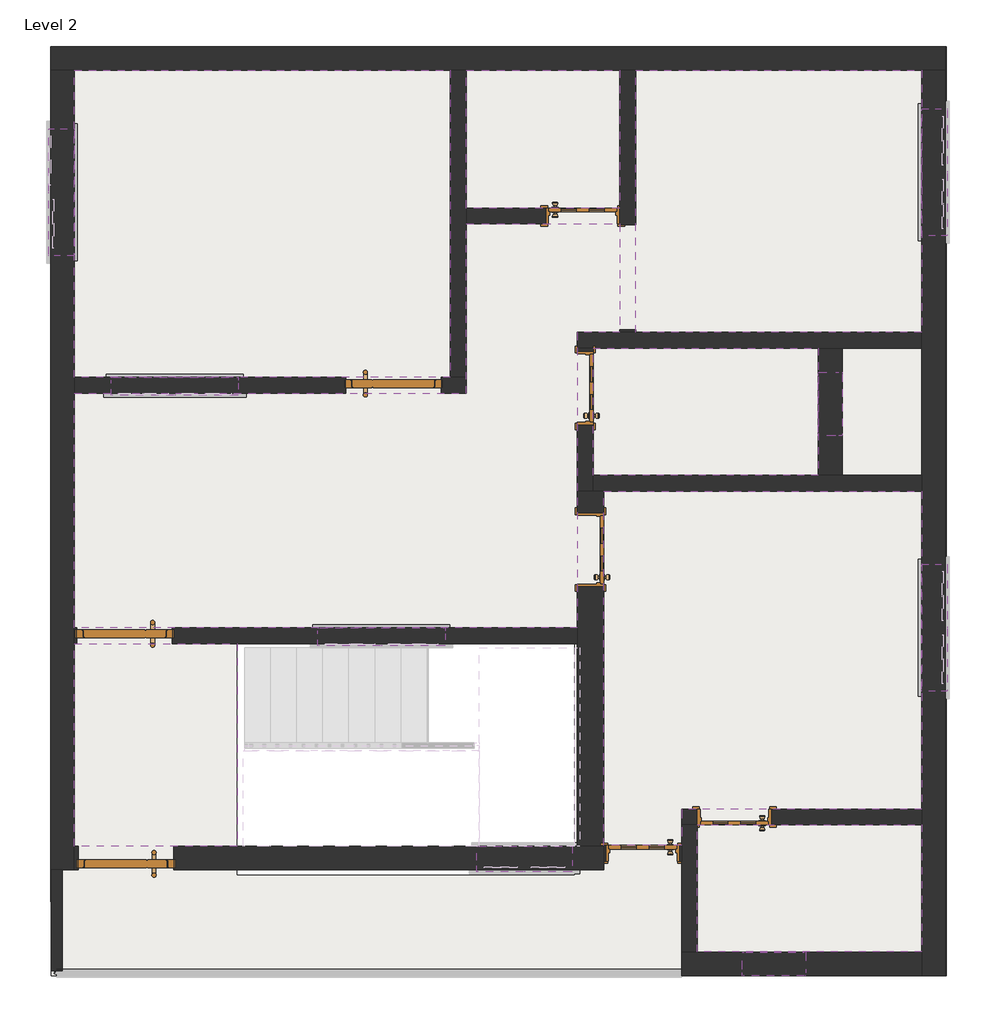
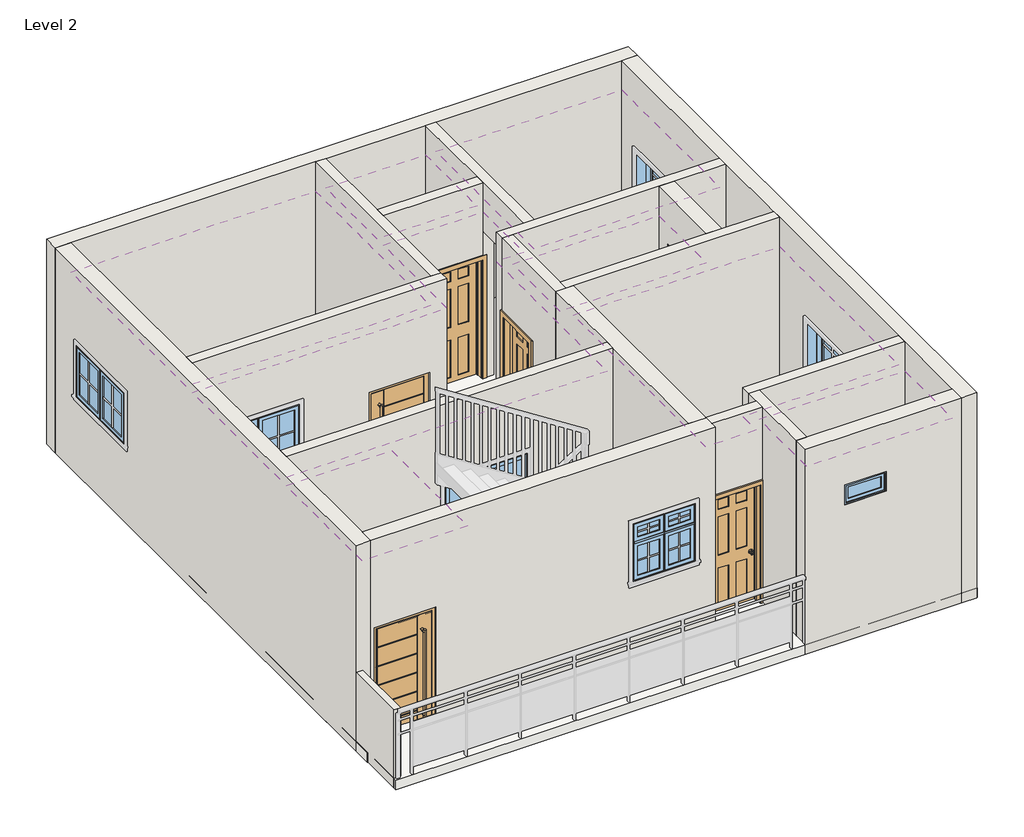
# One storey, part 1 of 2: 19 walls, 9 coverings, 8 doors, 8 windows, 1 slab.
"""IFC4 building model written with IfcOpenShell, lengths in millimetres."""

from ifc_helpers import new_model, si_unit, frame, origin, place, context, project, spatial, polyline, outline, extrude, faceted_brep, transform, mapped, element, save
from components import door_3_ad1505b7, door_3_abbf6f65, door_3_44036f4b, door_809e0d7a, door_c4e61f94, door_c896847d, m_fixed_2_dd9f9b20, m_window_awning_double_horizontal_4_8afcb0b2, m_window_awning_double_horizontal_4_cab21571, m_window_casement_double_awning_double_3_6fa9dbfe

model = new_model("IFC4")

# Units and contexts
model_context = context("Model", 3, world=origin())
ifc_project = project(units=[si_unit("LENGTHUNIT", "METRE", prefix="MILLI")], contexts=[model_context])

# Site, building, storey
site = spatial("IfcSite", under=ifc_project)
building = spatial("IfcBuilding", under=site)
storey = spatial("IfcBuildingStorey", under=building, Name="Level 2", Elevation=3200.4)

# Coverings
placement = place(None, origin())
element("IfcCovering", 1, ObjectType="Plain", at=placement, inside=storey, context=model_context, shape_type="SweptSolid", body=[
    extrude(outline(polyline([(-11429.8282945, 3413.9578397), (-7823.0282945, 3413.9578397), (-7823.0282945, 467.5578397), (-11429.8282945, 467.5578397), (-11429.8282945, 3413.9578397)])), frame((0.0, 0.0, 5943.6), z_axis=(0.0, 0.0, 1.0), x_axis=(1.0, 0.0, 0.0)), (0.0, 0.0, 1.0), 57.0),
])
element("IfcCovering", 2, ObjectType="Plain", at=placement, inside=storey, context=model_context, shape_type="SweptSolid", body=[
    extrude(outline(polyline([(-7670.6282945, 3413.9578397), (-6197.4282945, 3413.9578397), (-6197.4282945, 2093.1578397), (-7670.6282945, 2093.1578397), (-7670.6282945, 3413.9578397)])), frame((0.0, 0.0, 5943.6), z_axis=(0.0, 0.0, 1.0), x_axis=(1.0, 0.0, 0.0)), (0.0, 0.0, 1.0), 57.0),
])
element("IfcCovering", 3, ObjectType="Plain", at=placement, inside=storey, context=model_context, shape_type="SweptSolid", body=[
    extrude(outline(polyline([(-6045.0282945, 899.3578397), (-6045.0282945, 3413.9578397), (-3301.8282945, 3413.9578397), (-3301.8282945, 899.3578397), (-6045.0282945, 899.3578397)])), frame((0.0, 0.0, 5943.6), z_axis=(0.0, 0.0, 1.0), x_axis=(1.0, 0.0, 0.0)), (0.0, 0.0, 1.0), 57.0),
])
element("IfcCovering", 4, ObjectType="Plain", at=placement, inside=storey, context=model_context, shape_type="SweptSolid", body=[
    extrude(outline(polyline([(-11429.8282945, -1932.7421603), (-11429.8282945, 315.1578397), (-7670.6282945, 315.1578397), (-7670.6282945, 1940.7578397), (-6197.4282945, 1940.7578397), (-6197.4282945, 899.3578397), (-6603.8282945, 899.3578397), (-6603.8282945, -548.4421603), (-6603.8282945, -1932.7421603), (-11429.8282945, -1932.7421603)])), frame((0.0, 0.0, 5943.6), z_axis=(0.0, 0.0, 1.0), x_axis=(1.0, 0.0, 0.0)), (0.0, 0.0, 1.0), 57.0),
])
element("IfcCovering", 5, ObjectType="Plain", at=placement, inside=storey, context=model_context, shape_type="SweptSolid", body=[
    extrude(outline(polyline([(-6603.8282945, -2085.1421603), (-6603.8282945, -4028.2421603), (-6632.7282945, -4028.2421603), (-6632.7282945, -2085.1421603), (-6603.8282945, -2085.1421603)])), frame((0.0, 0.0, 5943.6), z_axis=(0.0, 0.0, 1.0), x_axis=(1.0, 0.0, 0.0)), (0.0, 0.0, 1.0), 57.0),
    extrude(outline(polyline([(-11429.8282945, -4028.2421603), (-11429.8282945, -2085.1421603), (-9869.3646777, -2085.1421603), (-9869.3646777, -4028.2421603), (-11429.8282945, -4028.2421603)])), frame((0.0, 0.0, 5943.6), z_axis=(0.0, 0.0, 1.0), x_axis=(1.0, 0.0, 0.0)), (0.0, 0.0, 1.0), 57.0),
])
element("IfcCovering", 6, ObjectType="Plain", at=placement, inside=storey, context=model_context, shape_type="SweptSolid", body=[
    extrude(outline(polyline([(-6349.8282945, -624.6421603), (-3301.8282945, -624.6421603), (-3301.8282945, -3672.6421603), (-5604.4329612, -3672.6421603), (-5604.4329612, -4021.3091242), (-6349.8282945, -4021.3091242), (-6349.8282945, -624.6421603)])), frame((0.0, 0.0, 5943.6), z_axis=(0.0, 0.0, 1.0), x_axis=(1.0, 0.0, 0.0)), (0.0, 0.0, 1.0), 57.0),
])
element("IfcCovering", 7, ObjectType="Plain", at=placement, inside=storey, context=model_context, shape_type="SweptSolid", body=[
    extrude(outline(polyline([(-6451.4282945, -472.2421603), (-6451.4282945, 746.9578397), (-4292.4282945, 746.9578397), (-4292.4282945, -472.2421603), (-6451.4282945, -472.2421603)])), frame((0.0, 0.0, 5943.6), z_axis=(0.0, 0.0, 1.0), x_axis=(1.0, 0.0, 0.0)), (0.0, 0.0, 1.0), 57.0),
])
element("IfcCovering", 8, ObjectType="Plain", at=placement, inside=storey, context=model_context, shape_type="SweptSolid", body=[
    extrude(outline(polyline([(-5452.0329612, -3825.0421603), (-3301.8282945, -3825.0421603), (-3301.8282945, -5044.2421603), (-5452.0329612, -5044.2421603), (-5452.0329612, -3825.0421603)])), frame((0.0, 0.0, 5943.6), z_axis=(0.0, 0.0, 1.0), x_axis=(1.0, 0.0, 0.0)), (0.0, 0.0, 1.0), 57.0),
])
element("IfcCovering", 9, ObjectType="Plain", at=placement, inside=storey, context=model_context, shape_type="SweptSolid", body=[
    extrude(outline(polyline([(-5452.0329612, -3825.0421603), (-3301.8282945, -3825.0421603), (-3301.8282945, -5044.2421603), (-5452.0329612, -5044.2421603), (-5452.0329612, -3825.0421603)])), frame((0.0, 0.0, 5943.6), z_axis=(0.0, 0.0, 1.0), x_axis=(1.0, 0.0, 0.0)), (0.0, 0.0, 1.0), 57.0),
])

# Doors
door_3_shape = door_3_ad1505b7(model_context)
element("IfcDoor", 10, ObjectType="3'", at=placement, inside=storey, context=model_context, shape_type="MappedRepresentation", body=[
    mapped(door_3_shape, transform((-8369.1282945, 391.3578397, 3200.4), x_axis=(1.0, 0.0, 0.0), y_axis=(0.0, 1.0, 0.0), z_axis=(0.0, 0.0, 1.0))),
])
door_3_2_shape = door_3_abbf6f65(model_context)
element("IfcDoor", 11, ObjectType="3'", at=placement, inside=storey, context=model_context, shape_type="MappedRepresentation", body=[
    mapped(door_3_2_shape, transform((-10934.5282945, -4142.5421603, 3200.4), x_axis=(-1.0, 0.0, 0.0), y_axis=(0.0, -1.0, 0.0), z_axis=(0.0, 0.0, 1.0))),
])
door_3_3_shape = door_3_44036f4b(model_context)
element("IfcDoor", 12, ObjectType="3'", at=placement, inside=storey, context=model_context, shape_type="MappedRepresentation", body=[
    mapped(door_3_3_shape, transform((-10947.2282945, -2008.9421603, 3200.4), x_axis=(-1.0, 0.0, 0.0), y_axis=(0.0, -1.0, 0.0), z_axis=(0.0, 0.0, 1.0))),
])
door_shape = door_809e0d7a(model_context)
element("IfcDoor", 13, ObjectType="M_Door-Interior-Single-6_Panel-Wood : 2'2\"", at=placement, inside=storey, context=model_context, shape_type="MappedRepresentation", body=[
    mapped(door_shape, transform((-6473.6532945, -1183.4421603, 3154.1554651), x_axis=(0.0, 1.0, 0.0), y_axis=(-1.0, 0.0, 0.0), z_axis=(0.0, 0.0, 1.0))),
])
door_2_shape = door_c4e61f94(model_context)
element("IfcDoor", 14, ObjectType="M_Door-Interior-Single-6_Panel-Wood : 2'2\"", at=placement, inside=storey, context=model_context, shape_type="MappedRepresentation", body=[
    mapped(door_2_shape, transform((-5096.8329612, -3752.0171603, 3200.4), x_axis=(-1.0, 0.0, 0.0), y_axis=(0.0, -1.0, 0.0), z_axis=(0.0, 0.0, 1.0))),
])
element("IfcDoor", 15, ObjectType="M_Door-Interior-Single-6_Panel-Wood : 2'2\"", at=placement, inside=storey, context=model_context, shape_type="MappedRepresentation", body=[
    mapped(door_2_shape, transform((-6552.6282945, 2020.1328397, 3200.4), x_axis=(1.0, 0.0, 0.0), y_axis=(0.0, 1.0, 0.0), z_axis=(0.0, 0.0, 1.0))),
])
door_4_shape = door_c896847d(model_context)
element("IfcDoor", 16, ObjectType="M_Door-Interior-Single-6_Panel-Wood : 2'2\"", at=placement, inside=storey, context=model_context, shape_type="MappedRepresentation", body=[
    mapped(door_4_shape, transform((-6524.4532945, 366.3578397, 3200.4), x_axis=(0.0, 1.0, 0.0), y_axis=(-1.0, 0.0, 0.0), z_axis=(0.0, 0.0, 1.0))),
])
element("IfcDoor", 17, ObjectType="M_Door-Interior-Single-6_Panel-Wood : 2'2\"", at=placement, inside=storey, context=model_context, shape_type="MappedRepresentation", body=[
    mapped(door_4_shape, transform((-5977.1306278, -4094.3341242, 3200.4), x_axis=(-1.0, 0.0, 0.0), y_axis=(0.0, -1.0, 0.0), z_axis=(0.0, 0.0, 1.0))),
])

# Slab
element("IfcSlab", 18, ObjectType="Generic 150mm", at=placement, inside=storey, context=model_context, shape_type="SweptSolid", body=[
    extrude(outline(polyline([(-3064.4329612, -5272.8421603), (-11649.6329612, -5272.8421603), (-11649.6329612, -4561.6421603), (-11658.4282945, -4561.6421603), (-11658.4282945, 3642.5578397), (-3064.4329612, 3642.5578397), (-3064.4329612, -5272.8421603)]), holes=[polyline([(-9869.3646777, -4303.0421603), (-6632.7282945, -4303.0421603), (-6632.7282945, -2085.1421603), (-9869.3646777, -2085.1421603), (-9869.3646777, -4303.0421603)])]), frame((0.0, 0.0, 3202.8), z_axis=(0.0, 0.0, 1.0), x_axis=(1.0, 0.0, 0.0)), (0.0, 0.0, 1.0), 150.0),
])

# Walls
element("IfcWall", 19, ObjectType="10\"", at=placement, inside=storey, context=model_context, shape_type="Brep", body=[
    faceted_brep([(-6349.8282945, -624.6421603, 6400.8), (-6349.8282945, -4021.3091242, 6400.8), (-6349.8282945, -4028.2421603, 6400.8), (-6349.8282945, -4028.2421603, 3200.4), (-6349.8282945, -4021.3091242, 3200.4), (-6349.8282945, -1538.6421603, 3200.4), (-6349.8282945, -1538.6421603, 5179.1554651), (-6349.8282945, -828.2421603, 5179.1554651), (-6349.8282945, -828.2421603, 3200.4), (-6349.8282945, -624.6421603, 3200.4), (-6603.8282945, -4028.2421603, 6400.8), (-6603.8282945, -2085.1421603, 6400.8), (-6603.8282945, -1932.7421603, 6400.8), (-6603.8282945, -624.6421603, 6400.8), (-6603.8282945, -624.6421603, 3200.4), (-6603.8282945, -828.2421603, 3200.4), (-6603.8282945, -828.2421603, 5179.1554651), (-6603.8282945, -1538.6421603, 5179.1554651), (-6603.8282945, -1538.6421603, 3200.4), (-6603.8282945, -1932.7421603, 3200.4), (-6603.8282945, -2085.1421603, 3200.4), (-6603.8282945, -4028.2421603, 3200.4), (-6451.4282945, -624.6421603, 3200.4), (-6451.4282945, -624.6421603, 6400.8)], [[[0, 1, 2, 3, 4, 5, 6, 7, 8, 9]], [[10, 11, 12, 13, 14, 15, 16, 17, 18, 19, 20, 21]], [[3, 21, 20, 19, 18, 5, 4]], [[14, 22, 9, 8, 15]], [[2, 1, 0, 23, 13, 12, 11, 10]], [[3, 2, 10, 21]], [[0, 9, 22, 14, 13, 23]], [[7, 16, 15, 8]], [[16, 7, 6, 17]], [[17, 6, 5, 18]]]),
])
element("IfcWall", 20, ObjectType="4\"", at=placement, inside=storey, context=model_context, shape_type="SweptSolid", body=[
    extrude(outline(polyline([(-11649.6329612, -5222.0421603), (-11649.6329612, -4256.8421603), (-11548.0329612, -4256.8421603), (-11548.0329612, -5222.0421603), (-11649.6329612, -5222.0421603)])), frame((0.0, 0.0, 3200.4), z_axis=(0.0, 0.0, 1.0), x_axis=(1.0, 0.0, 0.0)), (0.0, 0.0, 1.0), 1219.2),
])
element("IfcWall", 21, ObjectType="6\"", at=placement, inside=storey, context=model_context, shape_type="Brep", body=[
    faceted_brep([(-7670.6282945, 315.1578397, 6400.8), (-11429.8282945, 315.1578397, 6400.8), (-11429.8282945, 315.1578397, 3200.4), (-8826.3282945, 315.1578397, 3200.4), (-8826.3282945, 315.1578397, 5029.2), (-7911.9282945, 315.1578397, 5029.2), (-7911.9282945, 315.1578397, 3200.4), (-7670.6282945, 315.1578397, 3200.4), (-11074.2282945, 315.1578397, 5219.6), (-9855.0282945, 315.1578397, 5219.6), (-9855.0282945, 315.1578397, 4419.6), (-11074.2282945, 315.1578397, 4419.6), (-11429.8282945, 467.5578397, 6400.8), (-7823.0282945, 467.5578397, 6400.8), (-7670.6282945, 467.5578397, 6400.8), (-7670.6282945, 467.5578397, 3200.4), (-7823.0282945, 467.5578397, 3200.4), (-7911.9282945, 467.5578397, 3200.4), (-7911.9282945, 467.5578397, 5029.2), (-8826.3282945, 467.5578397, 5029.2), (-8826.3282945, 467.5578397, 3200.4), (-11429.8282945, 467.5578397, 3200.4), (-11074.2282945, 467.5578397, 5219.6), (-11074.2282945, 467.5578397, 4419.6), (-9855.0282945, 467.5578397, 4419.6), (-9855.0282945, 467.5578397, 5219.6), (-8826.3282945, 447.5578397, 3200.4), (-8841.3282945, 447.5578397, 3200.4), (-8841.3282945, 370.5578397, 3200.4), (-8826.3282945, 370.5578397, 3200.4), (-7911.9282945, 370.5578397, 3200.4), (-7896.9282945, 370.5578397, 3200.4), (-7896.9282945, 447.5578397, 3200.4), (-7911.9282945, 447.5578397, 3200.4), (-7911.9282945, 447.5578397, 5029.2), (-8826.3282945, 447.5578397, 5029.2), (-8826.3282945, 370.5578397, 5029.2), (-7911.9282945, 370.5578397, 5029.2), (-8841.3282945, 447.5578397, 5044.2), (-7896.9282945, 447.5578397, 5044.2), (-7896.9282945, 370.5578397, 5044.2), (-8841.3282945, 370.5578397, 5044.2)], [[[0, 1, 2, 3, 4, 5, 6, 7], [8, 9, 10, 11]], [[12, 13, 14, 15, 16, 17, 18, 19, 20, 21], [22, 23, 24, 25]], [[2, 21, 20, 26, 27, 28, 29, 3]], [[15, 7, 6, 30, 31, 32, 33, 17, 16]], [[1, 0, 14, 13, 12]], [[2, 1, 12, 21]], [[0, 7, 15, 14]], [[18, 34, 35, 19]], [[4, 36, 37, 5]], [[34, 18, 17, 33]], [[5, 37, 30, 6]], [[19, 35, 26, 20]], [[36, 4, 3, 29]], [[38, 39, 40, 41]], [[40, 39, 32, 31]], [[37, 36, 29, 28, 41, 40, 31, 30]], [[38, 41, 28, 27]], [[35, 34, 33, 32, 39, 38, 27, 26]], [[23, 22, 8, 11]], [[24, 23, 11, 10]], [[25, 24, 10, 9]], [[22, 25, 9, 8]]]),
])
element("IfcWall", 22, ObjectType="6\"", at=placement, inside=storey, context=model_context, shape_type="Brep", body=[
    faceted_brep([(-7670.6282945, 467.5578397, 3200.4), (-7670.6282945, 1940.7578397, 3200.4), (-7670.6282945, 2093.1578397, 3200.4), (-7670.6282945, 3413.9578397, 3200.4), (-7670.6282945, 3413.9578397, 6400.8), (-7670.6282945, 2093.1578397, 6400.8), (-7670.6282945, 1940.7578397, 6400.8), (-7670.6282945, 467.5578397, 6400.8), (-7823.0282945, 467.5578397, 3200.4), (-7823.0282945, 467.5578397, 6400.8), (-7823.0282945, 3413.9578397, 6400.8), (-7823.0282945, 3413.9578397, 3200.4)], [[[0, 1, 2, 3, 4, 5, 6, 7]], [[8, 9, 10, 11]], [[3, 2, 1, 0, 8, 11]], [[7, 6, 5, 4, 10, 9]], [[0, 7, 9, 8]], [[4, 3, 11, 10]]]),
])
element("IfcWall", 23, ObjectType="6\"", at=placement, inside=storey, context=model_context, shape_type="Brep", body=[
    faceted_brep([(-6197.4282945, 899.3578397, 3200.4), (-6197.4282945, 899.3578397, 6400.8), (-6197.4282945, 1940.7578397, 6400.8), (-6197.4282945, 2093.1578397, 6400.8), (-6197.4282945, 3413.9578397, 6400.8), (-6197.4282945, 3413.9578397, 3200.4), (-6197.4282945, 1930.784409, 3200.4), (-6197.4282945, 1930.784409, 5638.8), (-6197.4282945, 925.5690992, 5638.8), (-6197.4282945, 925.5690992, 3200.4), (-6045.0282945, 899.3578397, 6400.8), (-6045.0282945, 899.3578397, 3200.4), (-6045.0282945, 925.5690992, 3200.4), (-6045.0282945, 925.5690992, 5638.8), (-6045.0282945, 1930.784409, 5638.8), (-6045.0282945, 1930.784409, 3200.4), (-6045.0282945, 3413.9578397, 3200.4), (-6045.0282945, 3413.9578397, 6400.8)], [[[0, 1, 2, 3, 4, 5, 6, 7, 8, 9]], [[10, 11, 12, 13, 14, 15, 16, 17]], [[5, 16, 15, 6]], [[11, 0, 9, 12]], [[4, 3, 2, 1, 10, 17]], [[5, 4, 17, 16]], [[1, 0, 11, 10]], [[7, 14, 13, 8]], [[14, 7, 6, 15]], [[8, 13, 12, 9]]]),
])
element("IfcWall", 24, ObjectType="6\"", at=placement, inside=storey, context=model_context, shape_type="Brep", body=[
    faceted_brep([(-3301.8282945, 899.3578397, 3200.4), (-6045.0282945, 899.3578397, 3200.4), (-6197.4282945, 899.3578397, 3200.4), (-6603.8282945, 899.3578397, 3200.4), (-6603.8282945, 899.3578397, 6400.8), (-6197.4282945, 899.3578397, 6400.8), (-6045.0282945, 899.3578397, 6400.8), (-3301.8282945, 899.3578397, 6400.8), (-3301.8282945, 746.9578397, 3200.4), (-3301.8282945, 746.9578397, 6400.8), (-4063.8282945, 746.9578397, 6400.8), (-4292.4282945, 746.9578397, 6400.8), (-6451.4282945, 746.9578397, 6400.8), (-6603.8282945, 746.9578397, 6400.8), (-6603.8282945, 746.9578397, 3200.4), (-6451.4282945, 746.9578397, 3200.4), (-4292.4282945, 746.9578397, 3200.4), (-4063.8282945, 746.9578397, 3200.4)], [[[0, 1, 2, 3, 4, 5, 6, 7]], [[8, 9, 10, 11, 12, 13, 14, 15, 16, 17]], [[3, 2, 1, 0, 8, 17, 16, 15, 14]], [[7, 6, 5, 4, 13, 12, 11, 10, 9]], [[0, 7, 9, 8]], [[4, 3, 14, 13]]]),
])
element("IfcWall", 25, ObjectType="6\"", at=placement, inside=storey, context=model_context, shape_type="Brep", body=[
    faceted_brep([(-6603.8282945, -624.6421603, 6400.8), (-6603.8282945, 746.9578397, 6400.8), (-6603.8282945, 746.9578397, 3200.4), (-6603.8282945, 721.5578397, 3200.4), (-6603.8282945, 721.5578397, 5225.4), (-6603.8282945, 11.1578397, 5225.4), (-6603.8282945, 11.1578397, 3200.4), (-6603.8282945, -624.6421603, 3200.4), (-6451.4282945, 746.9578397, 6400.8), (-6451.4282945, -472.2421603, 6400.8), (-6451.4282945, -624.6421603, 6400.8), (-6451.4282945, -624.6421603, 3200.4), (-6451.4282945, -472.2421603, 3200.4), (-6451.4282945, 11.1578397, 3200.4), (-6451.4282945, 11.1578397, 5225.4), (-6451.4282945, 721.5578397, 5225.4), (-6451.4282945, 721.5578397, 3200.4), (-6451.4282945, 746.9578397, 3200.4)], [[[0, 1, 2, 3, 4, 5, 6, 7]], [[8, 9, 10, 11, 12, 13, 14, 15, 16, 17]], [[2, 17, 16, 3]], [[11, 7, 6, 13, 12]], [[1, 0, 10, 9, 8]], [[2, 1, 8, 17]], [[0, 7, 11, 10]], [[15, 4, 3, 16]], [[4, 15, 14, 5]], [[5, 14, 13, 6]]]),
])
element("IfcWall", 26, ObjectType="6\"", at=placement, inside=storey, context=model_context, shape_type="Brep", body=[
    faceted_brep([(-3301.8282945, -472.2421603, 3200.4), (-4063.8282945, -472.2421603, 3200.4), (-4292.4282945, -472.2421603, 3200.4), (-6451.4282945, -472.2421603, 3200.4), (-6451.4282945, -472.2421603, 6400.8), (-4292.4282945, -472.2421603, 6400.8), (-4063.8282945, -472.2421603, 6400.8), (-3301.8282945, -472.2421603, 6400.8), (-3301.8282945, -624.6421603, 3200.4), (-3301.8282945, -624.6421603, 6400.8), (-6349.8282945, -624.6421603, 6400.8), (-6451.4282945, -624.6421603, 6400.8), (-6451.4282945, -624.6421603, 3200.4), (-6349.8282945, -624.6421603, 3200.4)], [[[0, 1, 2, 3, 4, 5, 6, 7]], [[8, 9, 10, 11, 12, 13]], [[3, 2, 1, 0, 8, 13, 12]], [[7, 6, 5, 4, 11, 10, 9]], [[0, 7, 9, 8]], [[4, 3, 12, 11]]]),
])
element("IfcWall", 27, ObjectType="6\"", at=placement, inside=storey, context=model_context, shape_type="Brep", body=[
    faceted_brep([(-11429.8282945, -1932.7421603, 6400.8), (-6603.8282945, -1932.7421603, 6400.8), (-6603.8282945, -1932.7421603, 3200.4), (-10490.0282945, -1932.7421603, 3200.4), (-10490.0282945, -1932.7421603, 5029.2), (-11404.4282945, -1932.7421603, 5029.2), (-11404.4282945, -1932.7421603, 3200.4), (-11429.8282945, -1932.7421603, 3200.4), (-9093.0282945, -1932.7421603, 5219.6), (-9093.0282945, -1932.7421603, 4419.6), (-7873.8282945, -1932.7421603, 4419.6), (-7873.8282945, -1932.7421603, 5219.6), (-6603.8282945, -2085.1421603, 6400.8), (-11429.8282945, -2085.1421603, 6400.8), (-11429.8282945, -2085.1421603, 3200.4), (-11404.4282945, -2085.1421603, 3200.4), (-11404.4282945, -2085.1421603, 5029.2), (-10490.0282945, -2085.1421603, 5029.2), (-10490.0282945, -2085.1421603, 3200.4), (-6603.8282945, -2085.1421603, 3200.4), (-9093.0282945, -2085.1421603, 5219.6), (-7873.8282945, -2085.1421603, 5219.6), (-7873.8282945, -2085.1421603, 4419.6), (-9093.0282945, -2085.1421603, 4419.6), (-11404.4282945, -1952.7421603, 3200.4), (-11419.4282945, -1952.7421603, 3200.4), (-11419.4282945, -2029.7421603, 3200.4), (-11404.4282945, -2029.7421603, 3200.4), (-10490.0282945, -2029.7421603, 3200.4), (-10475.0282945, -2029.7421603, 3200.4), (-10475.0282945, -1952.7421603, 3200.4), (-10490.0282945, -1952.7421603, 3200.4), (-10490.0282945, -1952.7421603, 5029.2), (-11404.4282945, -1952.7421603, 5029.2), (-11404.4282945, -2029.7421603, 5029.2), (-10490.0282945, -2029.7421603, 5029.2), (-10475.0282945, -1952.7421603, 5044.2), (-10475.0282945, -2029.7421603, 5044.2), (-11419.4282945, -2029.7421603, 5044.2), (-11419.4282945, -1952.7421603, 5044.2)], [[[0, 1, 2, 3, 4, 5, 6, 7], [8, 9, 10, 11]], [[12, 13, 14, 15, 16, 17, 18, 19], [20, 21, 22, 23]], [[14, 7, 6, 24, 25, 26, 27, 15]], [[2, 19, 18, 28, 29, 30, 31, 3]], [[1, 0, 13, 12]], [[0, 7, 14, 13]], [[2, 1, 12, 19]], [[4, 32, 33, 5]], [[16, 34, 35, 17]], [[5, 33, 24, 6]], [[34, 16, 15, 27]], [[32, 4, 3, 31]], [[17, 35, 28, 18]], [[36, 37, 38, 39]], [[39, 38, 26, 25]], [[35, 34, 27, 26, 38, 37, 29, 28]], [[37, 36, 30, 29]], [[33, 32, 31, 30, 36, 39, 25, 24]], [[9, 8, 20, 23]], [[10, 9, 23, 22]], [[11, 10, 22, 21]], [[8, 11, 21, 20]]]),
])
element("IfcWall", 28, ObjectType="6\"", at=placement, inside=storey, context=model_context, shape_type="Brep", body=[
    faceted_brep([(-5604.4329612, -3672.6421603, 6400.8), (-3301.8282945, -3672.6421603, 6400.8), (-3301.8282945, -3672.6421603, 3200.4), (-4741.6329612, -3672.6421603, 3200.4), (-4741.6329612, -3672.6421603, 5225.4), (-5452.0329612, -3672.6421603, 5225.4), (-5452.0329612, -3672.6421603, 3200.4), (-5604.4329612, -3672.6421603, 3200.4), (-3301.8282945, -3825.0421603, 6400.8), (-5452.0329612, -3825.0421603, 6400.8), (-5604.4329612, -3825.0421603, 6400.8), (-5604.4329612, -3825.0421603, 3200.4), (-5452.0329612, -3825.0421603, 3200.4), (-5452.0329612, -3825.0421603, 5225.4), (-4741.6329612, -3825.0421603, 5225.4), (-4741.6329612, -3825.0421603, 3200.4), (-3301.8282945, -3825.0421603, 3200.4)], [[[0, 1, 2, 3, 4, 5, 6, 7]], [[8, 9, 10, 11, 12, 13, 14, 15, 16]], [[2, 16, 15, 3]], [[11, 7, 6, 12]], [[1, 0, 10, 9, 8]], [[2, 1, 8, 16]], [[0, 7, 11, 10]], [[5, 13, 12, 6]], [[13, 5, 4, 14]], [[14, 4, 3, 15]]]),
])
element("IfcWall", 29, ObjectType="6\"", at=placement, inside=storey, context=model_context, shape_type="Brep", body=[
    faceted_brep([(-5452.0329612, -5044.2421603, 3200.4), (-5452.0329612, -3825.0421603, 3200.4), (-5452.0329612, -3825.0421603, 5225.4), (-5452.0329612, -3825.0421603, 6400.8), (-5452.0329612, -5044.2421603, 6400.8), (-5604.4329612, -5044.2421603, 3200.4), (-5604.4329612, -5044.2421603, 6400.8), (-5604.4329612, -4173.7091242, 6400.8), (-5604.4329612, -4021.3091242, 6400.8), (-5604.4329612, -3825.0421603, 6400.8), (-5604.4329612, -3825.0421603, 3200.4), (-5604.4329612, -4021.3091242, 3200.4), (-5604.4329612, -4173.7091242, 3200.4)], [[[0, 1, 2, 3, 4]], [[5, 6, 7, 8, 9, 10, 11, 12]], [[1, 0, 5, 12, 11, 10]], [[4, 3, 9, 8, 7, 6]], [[3, 2, 1, 10, 9]], [[0, 4, 6, 5]]]),
])
element("IfcWall", 30, ObjectType="6\"", at=placement, inside=storey, context=model_context, shape_type="SweptSolid", body=[
    extrude(outline(polyline([(6400.8, -6197.4282945), (6400.8, -7670.6282945), (3200.4, -7670.6282945), (3200.4, -6907.8282945), (5225.4, -6907.8282945), (5225.4, -6197.4282945), (6400.8, -6197.4282945)])), frame((0.0, 1940.7578397, 0.0), z_axis=(0.0, 1.0, 0.0), x_axis=(0.0, 0.0, 1.0)), (0.0, 0.0, 1.0), 152.4),
])
element("IfcWall", 31, ObjectType="6\"", at=placement, inside=storey, context=model_context, shape_type="Brep", body=[
    faceted_brep([(-5604.4329612, -4173.7091242, 6400.8), (-6349.8282945, -4173.7091242, 6400.8), (-6349.8282945, -4173.7091242, 3200.4), (-6332.3306278, -4173.7091242, 3200.4), (-6332.3306278, -4173.7091242, 5225.4), (-5621.9306278, -4173.7091242, 5225.4), (-5621.9306278, -4173.7091242, 3200.4), (-5604.4329612, -4173.7091242, 3200.4), (-6349.8282945, -4021.3091242, 6400.8), (-5604.4329612, -4021.3091242, 6400.8), (-5604.4329612, -4021.3091242, 3200.4), (-5621.9306278, -4021.3091242, 3200.4), (-5621.9306278, -4021.3091242, 5225.4), (-6332.3306278, -4021.3091242, 5225.4), (-6332.3306278, -4021.3091242, 3200.4), (-6349.8282945, -4021.3091242, 3200.4), (-6349.8282945, -4028.2421603, 3200.4), (-6349.8282945, -4028.2421603, 6400.8)], [[[0, 1, 2, 3, 4, 5, 6, 7]], [[8, 9, 10, 11, 12, 13, 14, 15]], [[2, 16, 15, 14, 3]], [[10, 7, 6, 11]], [[1, 0, 9, 8, 17]], [[2, 1, 17, 8, 15, 16]], [[0, 7, 10, 9]], [[13, 4, 3, 14]], [[4, 13, 12, 5]], [[5, 12, 11, 6]]]),
])
element("IfcWall", 32, ObjectType="9\"", at=placement, inside=storey, context=model_context, shape_type="Brep", body=[
    faceted_brep([(-11658.4282945, 3413.9578397, 3200.4), (-11429.8282945, 3413.9578397, 3200.4), (-7823.0282945, 3413.9578397, 3200.4), (-7670.6282945, 3413.9578397, 3200.4), (-6197.4282945, 3413.9578397, 3200.4), (-6045.0282945, 3413.9578397, 3200.4), (-3301.8282945, 3413.9578397, 3200.4), (-3073.2282945, 3413.9578397, 3200.4), (-3073.2282945, 3413.9578397, 6400.8), (-3301.8282945, 3413.9578397, 6400.8), (-6045.0282945, 3413.9578397, 6400.8), (-6197.4282945, 3413.9578397, 6400.8), (-7670.6282945, 3413.9578397, 6400.8), (-7823.0282945, 3413.9578397, 6400.8), (-11429.8282945, 3413.9578397, 6400.8), (-11658.4282945, 3413.9578397, 6400.8), (-11658.4282945, 3642.5578397, 3200.4), (-11658.4282945, 3642.5578397, 6400.8), (-3073.2282945, 3642.5578397, 6400.8), (-3073.2282945, 3642.5578397, 3200.4)], [[[0, 1, 2, 3, 4, 5, 6, 7, 8, 9, 10, 11, 12, 13, 14, 15]], [[16, 17, 18, 19]], [[7, 6, 5, 4, 3, 2, 1, 0, 16, 19]], [[15, 14, 13, 12, 11, 10, 9, 8, 18, 17]], [[8, 7, 19, 18]], [[0, 15, 17, 16]]]),
])
element("IfcWall", 33, ObjectType="9\"", at=placement, inside=storey, context=model_context, shape_type="Brep", body=[
    faceted_brep([(-3301.8282945, 3413.9578397, 3200.4), (-3301.8282945, 899.3578397, 3200.4), (-3301.8282945, 746.9578397, 3200.4), (-3301.8282945, -472.2421603, 3200.4), (-3301.8282945, -624.6421603, 3200.4), (-3301.8282945, -3672.6421603, 3200.4), (-3301.8282945, -3825.0421603, 3200.4), (-3301.8282945, -5044.2421603, 3200.4), (-3301.8282945, -5272.8421603, 3200.4), (-3301.8282945, -5272.8421603, 6400.8), (-3301.8282945, -5044.2421603, 6400.8), (-3301.8282945, -3825.0421603, 6400.8), (-3301.8282945, -3672.6421603, 6400.8), (-3301.8282945, -624.6421603, 6400.8), (-3301.8282945, -472.2421603, 6400.8), (-3301.8282945, 746.9578397, 6400.8), (-3301.8282945, 899.3578397, 6400.8), (-3301.8282945, 3413.9578397, 6400.8), (-3301.8282945, -2542.3421603, 5219.6), (-3301.8282945, -2542.3421603, 4419.6), (-3301.8282945, -1323.1421603, 4419.6), (-3301.8282945, -1323.1421603, 5219.6), (-3301.8282945, 1826.4578397, 5219.6), (-3301.8282945, 1826.4578397, 4419.6), (-3301.8282945, 3045.6578397, 4419.6), (-3301.8282945, 3045.6578397, 5219.6), (-3073.2282945, 3413.9578397, 3200.4), (-3073.2282945, 3413.9578397, 6400.8), (-3073.2282945, -5272.8421603, 6400.8), (-3073.2282945, -5272.8421603, 3200.4), (-3073.2282945, -2542.3421603, 5219.6), (-3073.2282945, -1323.1421603, 5219.6), (-3073.2282945, -1323.1421603, 4419.6), (-3073.2282945, -2542.3421603, 4419.6), (-3073.2282945, 1826.4578397, 5219.6), (-3073.2282945, 3045.6578397, 5219.6), (-3073.2282945, 3045.6578397, 4419.6), (-3073.2282945, 1826.4578397, 4419.6)], [[[0, 1, 2, 3, 4, 5, 6, 7, 8, 9, 10, 11, 12, 13, 14, 15, 16, 17], [18, 19, 20, 21], [22, 23, 24, 25]], [[26, 27, 28, 29], [30, 31, 32, 33], [34, 35, 36, 37]], [[8, 7, 6, 5, 4, 3, 2, 1, 0, 26, 29]], [[17, 16, 15, 14, 13, 12, 11, 10, 9, 28, 27]], [[0, 17, 27, 26]], [[9, 8, 29, 28]], [[19, 18, 30, 33]], [[20, 19, 33, 32]], [[21, 20, 32, 31]], [[18, 21, 31, 30]], [[23, 22, 34, 37]], [[24, 23, 37, 36]], [[25, 24, 36, 35]], [[22, 25, 35, 34]]]),
])
element("IfcWall", 34, ObjectType="9\"", at=placement, inside=storey, context=model_context, shape_type="Brep", body=[
    faceted_brep([(-3301.8282945, -5044.2421603, 3200.4), (-5452.0329612, -5044.2421603, 3200.4), (-5604.4329612, -5044.2421603, 3200.4), (-5604.4329612, -5044.2421603, 6400.8), (-5452.0329612, -5044.2421603, 6400.8), (-3301.8282945, -5044.2421603, 6400.8), (-4410.6329612, -5044.2421603, 5334.0), (-4410.6329612, -5044.2421603, 5638.8), (-5020.2329612, -5044.2421603, 5638.8), (-5020.2329612, -5044.2421603, 5334.0), (-3301.8282945, -5272.8421603, 3200.4), (-3301.8282945, -5272.8421603, 6400.8), (-5604.4329612, -5272.8421603, 6400.8), (-5604.4329612, -5272.8421603, 3200.4), (-4410.6329612, -5272.8421603, 5334.0), (-5020.2329612, -5272.8421603, 5334.0), (-5020.2329612, -5272.8421603, 5638.8), (-4410.6329612, -5272.8421603, 5638.8)], [[[0, 1, 2, 3, 4, 5], [6, 7, 8, 9]], [[10, 11, 12, 13], [14, 15, 16, 17]], [[2, 1, 0, 10, 13]], [[5, 4, 3, 12, 11]], [[0, 5, 11, 10]], [[7, 6, 14, 17]], [[8, 7, 17, 16]], [[9, 8, 16, 15]], [[6, 9, 15, 14]], [[3, 2, 13, 12]]]),
])
element("IfcWall", 35, ObjectType="9\"", at=placement, inside=storey, context=model_context, shape_type="Brep", body=[
    faceted_brep([(-11429.8282945, -4256.8421603, 6400.8), (-11429.8282945, -4256.8421603, 3200.4), (-11429.8282945, -4028.2421603, 3200.4), (-11429.8282945, -2085.1421603, 3200.4), (-11429.8282945, -1932.7421603, 3200.4), (-11429.8282945, 315.1578397, 3200.4), (-11429.8282945, 467.5578397, 3200.4), (-11429.8282945, 3413.9578397, 3200.4), (-11429.8282945, 3413.9578397, 6400.8), (-11429.8282945, 467.5578397, 6400.8), (-11429.8282945, 315.1578397, 6400.8), (-11429.8282945, -1932.7421603, 6400.8), (-11429.8282945, -2085.1421603, 6400.8), (-11429.8282945, -4028.2421603, 6400.8), (-11429.8282945, 2855.1578397, 5219.6), (-11429.8282945, 2855.1578397, 4419.6), (-11429.8282945, 1635.9578397, 4419.6), (-11429.8282945, 1635.9578397, 5219.6), (-11658.4282945, -4256.8421603, 3200.4), (-11658.4282945, -4256.8421603, 6400.8), (-11658.4282945, 3413.9578397, 6400.8), (-11658.4282945, 3413.9578397, 3200.4), (-11658.4282945, 2855.1578397, 5219.6), (-11658.4282945, 1635.9578397, 5219.6), (-11658.4282945, 1635.9578397, 4419.6), (-11658.4282945, 2855.1578397, 4419.6), (-11548.0329612, -4256.8421603, 3200.4), (-11649.6329612, -4256.8421603, 3200.4)], [[[0, 1, 2, 3, 4, 5, 6, 7, 8, 9, 10, 11, 12, 13], [14, 15, 16, 17]], [[18, 19, 20, 21], [22, 23, 24, 25]], [[7, 6, 5, 4, 3, 2, 1, 26, 27, 18, 21]], [[0, 13, 12, 11, 10, 9, 8, 20, 19]], [[8, 7, 21, 20]], [[0, 19, 18, 27, 26, 1]], [[15, 14, 22, 25]], [[16, 15, 25, 24]], [[17, 16, 24, 23]], [[14, 17, 23, 22]]]),
])
element("IfcWall", 36, ObjectType="9\"", at=placement, inside=storey, context=model_context, shape_type="Brep", body=[
    faceted_brep([(-11429.8282945, -4028.2421603, 6400.8), (-6603.8282945, -4028.2421603, 6400.8), (-6349.8282945, -4028.2421603, 6400.8), (-6349.8282945, -4028.2421603, 3200.4), (-6603.8282945, -4028.2421603, 3200.4), (-10477.3282945, -4028.2421603, 3200.4), (-10477.3282945, -4028.2421603, 5029.2), (-11391.7282945, -4028.2421603, 5029.2), (-11391.7282945, -4028.2421603, 3200.4), (-11429.8282945, -4028.2421603, 3200.4), (-7569.0282945, -4028.2421603, 5319.6), (-7569.0282945, -4028.2421603, 4419.6), (-6654.6282945, -4028.2421603, 4419.6), (-6654.6282945, -4028.2421603, 5319.6), (-6349.8282945, -4256.8421603, 6400.8), (-11429.8282945, -4256.8421603, 6400.8), (-11429.8282945, -4256.8421603, 3200.4), (-11391.7282945, -4256.8421603, 3200.4), (-11391.7282945, -4256.8421603, 5029.2), (-10477.3282945, -4256.8421603, 5029.2), (-10477.3282945, -4256.8421603, 3200.4), (-6349.8282945, -4256.8421603, 3200.4), (-7569.0282945, -4256.8421603, 5319.6), (-6654.6282945, -4256.8421603, 5319.6), (-6654.6282945, -4256.8421603, 4419.6), (-7569.0282945, -4256.8421603, 4419.6), (-11391.7282945, -4159.8421603, 3200.4), (-11406.7282945, -4159.8421603, 3200.4), (-11406.7282945, -4236.8421603, 3200.4), (-11391.7282945, -4236.8421603, 3200.4), (-6349.8282945, -4173.7091242, 3200.4), (-10477.3282945, -4236.8421603, 3200.4), (-10462.3282945, -4236.8421603, 3200.4), (-10462.3282945, -4159.8421603, 3200.4), (-10477.3282945, -4159.8421603, 3200.4), (-6349.8282945, -4173.7091242, 6400.8), (-11391.7282945, -4236.8421603, 5029.2), (-10477.3282945, -4236.8421603, 5029.2), (-10477.3282945, -4159.8421603, 5029.2), (-11391.7282945, -4159.8421603, 5029.2), (-10462.3282945, -4236.8421603, 5044.2), (-11406.7282945, -4236.8421603, 5044.2), (-11406.7282945, -4159.8421603, 5044.2), (-10462.3282945, -4159.8421603, 5044.2)], [[[0, 1, 2, 3, 4, 5, 6, 7, 8, 9], [10, 11, 12, 13]], [[14, 15, 16, 17, 18, 19, 20, 21], [22, 23, 24, 25]], [[16, 9, 8, 26, 27, 28, 29, 17]], [[3, 30, 21, 20, 31, 32, 33, 34, 5, 4]], [[2, 1, 0, 15, 14, 35]], [[3, 2, 35, 14, 21, 30]], [[9, 16, 15, 0]], [[18, 36, 37, 19]], [[6, 38, 39, 7]], [[36, 18, 17, 29]], [[7, 39, 26, 8]], [[19, 37, 31, 20]], [[38, 6, 5, 34]], [[40, 41, 42, 43]], [[42, 41, 28, 27]], [[39, 38, 34, 33, 43, 42, 27, 26]], [[40, 43, 33, 32]], [[37, 36, 29, 28, 41, 40, 32, 31]], [[11, 10, 22, 25]], [[12, 11, 25, 24]], [[13, 12, 24, 23]], [[10, 13, 23, 22]]]),
])
element("IfcWall", 37, ObjectType="9\"", at=placement, inside=storey, context=model_context, shape_type="SweptSolid", body=[
    extrude(outline(polyline([(746.9578397, 3200.4), (-472.2421603, 3200.4), (-472.2421603, 6400.8), (746.9578397, 6400.8), (746.9578397, 3200.4)]), holes=[polyline([(518.3578397, 5334.0), (518.3578397, 5638.8), (-91.2421603, 5638.8), (-91.2421603, 5334.0), (518.3578397, 5334.0)])]), frame((-4292.4282945, 0.0, 0.0), z_axis=(1.0, 0.0, 0.0), x_axis=(0.0, 1.0, 0.0)), (0.0, 0.0, 1.0), 228.6),
])

# Windows
m_fixed_2_shape = m_fixed_2_dd9f9b20(model_context)
element("IfcWindow", 38, ObjectType="M_Fixed : 2'", at=placement, inside=storey, context=model_context, shape_type="MappedRepresentation", body=[
    mapped(m_fixed_2_shape, transform((-4715.4329612, -5145.5421603, 4419.0), x_axis=(-1.0, 0.0, 0.0), y_axis=(0.0, -1.0, 0.0), z_axis=(0.0, 0.0, 1.0))),
])
element("IfcWindow", 39, ObjectType="M_Fixed : 2'", at=placement, inside=storey, context=model_context, shape_type="MappedRepresentation", body=[
    mapped(m_fixed_2_shape, transform((-4191.1282945, 213.5578397, 4419.0), x_axis=(0.0, -1.0, 0.0), y_axis=(1.0, 0.0, 0.0), z_axis=(0.0, 0.0, 1.0))),
])
m_window_awning_double_horizontal_4_shape = m_window_awning_double_horizontal_4_8afcb0b2(model_context)
element("IfcWindow", 40, ObjectType="M_Window-Awning-Double-Horizontal : 4'", at=placement, inside=storey, context=model_context, shape_type="MappedRepresentation", body=[
    mapped(m_window_awning_double_horizontal_4_shape, transform((-3187.5282945, -1932.7421603, 3519.6), x_axis=(0.0, -1.0, 0.0), y_axis=(1.0, 0.0, 0.0), z_axis=(0.0, 0.0, 1.0))),
])
element("IfcWindow", 41, ObjectType="M_Window-Awning-Double-Horizontal : 4'", at=placement, inside=storey, context=model_context, shape_type="MappedRepresentation", body=[
    mapped(m_window_awning_double_horizontal_4_shape, transform((-3187.5282945, 2436.0578397, 3519.6), x_axis=(0.0, -1.0, 0.0), y_axis=(1.0, 0.0, 0.0), z_axis=(0.0, 0.0, 1.0))),
])
element("IfcWindow", 42, ObjectType="M_Window-Awning-Double-Horizontal : 4'", at=placement, inside=storey, context=model_context, shape_type="MappedRepresentation", body=[
    mapped(m_window_awning_double_horizontal_4_shape, transform((-11544.1282945, 2245.5578397, 3519.6), x_axis=(0.0, 1.0, 0.0), y_axis=(-1.0, 0.0, 0.0), z_axis=(0.0, 0.0, 1.0))),
])
m_window_awning_double_horizontal_4_2_shape = m_window_awning_double_horizontal_4_cab21571(model_context)
element("IfcWindow", 43, ObjectType="M_Window-Awning-Double-Horizontal : 4'", at=placement, inside=storey, context=model_context, shape_type="MappedRepresentation", body=[
    mapped(m_window_awning_double_horizontal_4_2_shape, transform((-10464.6282945, 391.3578397, 3519.6), x_axis=(-1.0, 0.0, 0.0), y_axis=(0.0, -1.0, 0.0), z_axis=(0.0, 0.0, 1.0))),
])
element("IfcWindow", 44, ObjectType="M_Window-Awning-Double-Horizontal : 4'", at=placement, inside=storey, context=model_context, shape_type="MappedRepresentation", body=[
    mapped(m_window_awning_double_horizontal_4_2_shape, transform((-8483.4282945, -2008.9421603, 3519.6), x_axis=(-1.0, 0.0, 0.0), y_axis=(0.0, -1.0, 0.0), z_axis=(0.0, 0.0, 1.0))),
])
m_window_casement_double_awning_double_3_shape = m_window_casement_double_awning_double_3_6fa9dbfe(model_context)
element("IfcWindow", 45, ObjectType="M_Window-Casement-Double-Awning-Double : 3'", at=placement, inside=storey, context=model_context, shape_type="MappedRepresentation", body=[
    mapped(m_window_casement_double_awning_double_3_shape, transform((-7111.8282945, -4142.5421603, 3519.6), x_axis=(-1.0, 0.0, 0.0), y_axis=(0.0, -1.0, 0.0), z_axis=(0.0, 0.0, 1.0))),
])

save(model, "model.ifc")

# Revit data of these elements
# Type "Plain"
#   built-in parameter 1002203 = 1 (stored number, unit not read)
#   built-in parameter 1002202 = 1 (stored number, unit not read)
#   Layers, outside or top first: 0' - 1.77165" "Metal Stud Layer" (function 1); 0' - 0.47244" "Gypsum Wall Board" (function 1)
# Type "3'"
#   Type Mark = "41"
#   Water resistance = "up to Class E900, EN 12208:2001"
#   Uniclass2015Version = "v1.21"
#   Uniclass2015Reference = "Ss_25_30_20_30"
#   Uniclass2015Description = "Frame and door leaf system"
#   URL = "www.aluprof.com"
#   Type IFC Predefined Type = "USERDEFINED"
#   Right-hand / Left-hand door [instance default] = ""
#   Resistance to wind load = "up to Class C5/B5, EN 12210:2001"
#   Insert type = "ST"
#   Hardware [instance default] = ""
#   Product page = "https://aluprof.com/en/architects/offer/window-and-door-systems/panel-doors#visualisation"
#   Operation = "SinglePanelOutwardOpening"
#   Opening type = "Outward"
#   NBSReference = "25-50-20/125"
#   NBSDescription = "Frame and door leaf system"
#   Important = "The actual acceptable construction dimensions are dependent on the selection of profiles and hardware, glazing type, construction weight and the construction’s operating conditions. These should be determined by a suitably qualified person, and using ALUPROF’s calculation software"
#   IfcExportType = "USERDEFINED"
#   IfcExportAs = "IfcDoorType"
#   Handle type [instance default] = ""
#   Manufacturer = "ALUPROF SA"
#   Export Type to IFC As = "IfcDoorType"
#   Door sill type [instance default] = ""
#   Description = "External single-leaf panel door outward opening"
#   Model = "MB-86 ST Panel Door AD07"
#   Content of the recyclate in the material = "69.2%"
#   COBie.Type.WarrantyDurationParts = ""
#   COBie.Type.Name = ""
#   COBie.Type.Manufacturer = "ALUPROF SA"
#   COBie.Space.Name = ""
#   COBie.Floor.Name = ""
#   COBie.Facility.Name = ""
#   COBie.CreatedOn = ""
#   COBie.Component.WarrantyStartDate = ""
#   COBie.Component.Name = "MB-86 ST Panel Door AD07"
#   Burglar resistance = "RC2"
#   Air permeability = "up to Class 4, EN 12207:2001"
#   Width of the active leaf = 2' - 8.17717"
#   Placement in wall = 0' - 0.7874"
#   Thickness = 0' - 3.0315"
#   Height of the opening sash = 5' - 9.44094"
#   Handle Offset = 3' - 5.33858"
#   Rough Height = 6' - 2.40945"
#   Rough Width = 3' - 1.1811"
#   Height = 6' - 0"
#   Width = 3' - 0"
#   Construction depth = 0' - 3.0315"
#   Clear opening width = 2' - 3.94882"
#   Clear opening height = 5' - 8.47638"
#   Height of the array = 0' - 11.08136"
#   Schedule No. [instance default] = 1
#   Handrail [instance default] = yes
#   IsExternal = yes
#   Handle [instance default] = no
#   Door closer [instance default] = no
#   Function = 1
#   COBie.Type = yes
#   COBie = yes
#   Access control [instance default] = no
#   Panel = element 371215
#   Wall Closure = (empty or 0)
# Type "M_Door-Interior-Single-6_Panel-Wood : 2'2\""
#   Type Mark = "47"
#   Assembly Code = "C1020300"
#   Analytic Construction = "Wooden"
#   Top Rail = 0' - 4.72441"
#   Top Panel = 0' - 6.01181"
#   Thickness = 0' - 1.37795"
#   Thermal Resistance (R) = 0.455703 (m²·K)/W
#   Swing Angle [instance default] = 90.00°
#   Stiles = 0' - 4.72441"
#   Rough Width = 2' - 3.9685"
#   Rough Height = 6' - 7.72441"
#   Mullion = 0' - 4.52756"
#   Lock Rail = 0' - 7.87402"
#   Intermediate Rail = 0' - 4.52756"
#   Height = 6' - 6.74016"
#   Width = 2' - 2"
#   Heat Transfer Coefficient (U) = 2.19465 W/(m²·K)
#   Bottom Rail = 0' - 9.05512"
#   Trim Material = Cherry
#   Panel Material = Cherry
#   Frame Material = Cherry
#   Door Handle Material = Aluminum
#   Visual Light Transmittance = 0
#   Solar Heat Gain Coefficient = 0
#   Wall Closure = (empty or 0)
#   Function = (empty or 0)
# Type "Generic 150mm"
#   Function = 0
#   Layers, outside or top first: 0' - 5.90551" no material (function 1)
# Type "10\""
#   Layers, outside or top first: 0' - 10" no material (function 1)
# Type "4\""
#   Layers, outside or top first: 0' - 4" no material (function 1)
# Type "6\""
#   Layers, outside or top first: 0' - 6" no material (function 1)
# Type "9\""
#   Layers, outside or top first: 0' - 9" no material (function 1)
# Type "M_Fixed : 2'"
#   Type Mark = "32"
#   Construction Type Id = "GSP4R"
#   Analytic Construction = "1/8 in Pilkington single glazing"
#   Visual Light Transmittance = 0.9
#   Thermal Resistance (R) = 0.271106 (m²·K)/W
#   Solar Heat Gain Coefficient = 0.78
#   Heat Transfer Coefficient (U) = 3.6886 W/(m²·K)
#   Height = 1' - 0"
#   Default Sill Height = 3' - 0.02362"
#   Width = 2' - 0"
#   Window Inset = 0' - 0.74803"
#   Define Thermal Properties by = 1
#   Frame Exterior Material = Sash
#   Frame Interior Material = Sash
#   Glass Pane Material = Glass
#   Sash = Sash
#   Wall Closure = (empty or 0)
# Type "M_Window-Awning-Double-Horizontal : 4'"
#   Type Mark = "28"
#   Fire Rating = "0.5h"
#   Assembly Code = "B2020100"
#   Analytic Construction = "Double glazing - domestic"
#   Window Inset [instance default] = 0' - 0"
#   Wall Thickness [instance default] = 0' - 5.90551"
#   Interior Wall Closure [instance default] = 0' - 2.15551"
#   Half Width = 2' - 0"
#   Visual Light Transmittance = 0.81
#   Thermal Resistance (R) = 0.319569 (m²·K)/W
#   Solar Heat Gain Coefficient = 0.76
#   Rough Width = 4' - 0.59055"
#   Rough Height = 2' - 8.08661"
#   Height = 2' - 7.49606"
#   Heat Transfer Coefficient (U) = 3.12929 W/(m²·K)
#   Frame Extension [instance default] = 0' - 0 1/4"
#   Exterior Wall Closure [instance default] = 0' - 1 1/4"
#   Extension Jamb [instance default] = 0' - 2.15551"
#   Default Sill Height = 2' - 11.43307"
#   Width = 4' - 0"
#   Muntin Visibility = yes
#   Interior Trim Visibility [instance default] = yes
#   Exterior Trim Visibility [instance default] = yes
#   Extension Jamb Visibility [instance default] = yes
#   Interior Trim Material = Wood - Stained
#   Muntin Pattern = M_Muntin Pattern_2x2 : M_Muntin Pattern_2x2
#   Interior Trim = M_Trim-Window-Interior-Flat : Picture Frame
#   Interior Frame Material = Wood - Stained
#   Glass Panel Material = Glass
#   Exterior Trim Material = Clad - White
#   Exterior Trim = M_Trim-Window-Exterior-Flat : with Sill
#   Exterior Frame Material = Clad - White
#   Wall Closure = (empty or 0)
# Type "M_Window-Casement-Double-Awning-Double : 3'"
#   Type Mark = "31"
#   Fire Rating = "0.5h"
#   Assembly Code = "B2020100"
#   Analytic Construction = "Double glazing - domestic"
#   Window Inset [instance default] = 0' - 0"
#   Wall Thickness [instance default] = 0' - 5.90551"
#   Interior Wall Closure [instance default] = 0' - 2.15551"
#   Half Width = 1' - 6"
#   Visual Light Transmittance = 0.81
#   Transom Height = 0' - 11.81102"
#   Thermal Resistance (R) = 0.319569 (m²·K)/W
#   Solar Heat Gain Coefficient = 0.76
#   Rough Width = 3' - 0.59055"
#   Rough Height = 3' - 0.02362"
#   Open Window Height = 1' - 11.62205"
#   Frame Extension [instance default] = 0' - 0 1/4"
#   Height = 2' - 11.43307"
#   Heat Transfer Coefficient (U) = 3.12929 W/(m²·K)
#   Exterior Wall Closure [instance default] = 0' - 1.25197"
#   Extension Jamb [instance default] = 0' - 2.15551"
#   Default Sill Height = 2' - 11.43307"
#   Width = 3' - 0"
#   Top Muntin Visibility = yes
#   Bottom Muntin Visibility = yes
#   Interior Trim Visibility [instance default] = yes
#   Exterior Trim Visibility [instance default] = yes
#   Extension Jamb Visibility [instance default] = yes
#   Interior Trim Material = Wood - Stained
#   Muntin Pattern = M_Muntin Pattern_2x2 : M_Muntin Pattern_2x2
#   Interior Trim = M_Trim-Window-Interior-Flat : Picture Frame
#   Interior Frame Material = Wood - Stained
#   Glass Panel Material = Glass
#   Exterior Trim Material = Clad - White
#   Exterior Trim = M_Trim-Window-Exterior-Flat : with Sill
#   Exterior Frame Material = Clad - White
#   Wall Closure = (empty or 0)
# Elements 1, 2, 3, 4, 5, 6, 7, 8, 9 (IfcCovering, "Plain")
#   Height Offset From Level = 9' - 0"
#   Phase Created = New Construction
#   Materials on its faces: "Gypsum Wall Board", "Metal Stud Layer"
# Elements 10, 11, 12 (IfcDoor, "3'")
#   Right-hand / Left-hand door = ""
#   Hardware = ""
#   Handle type = ""
#   Door sill type = ""
#   Schedule No. = 1
#   Handrail = yes
#   Handle = no
#   Door closer = no
#   Access control = no
#   Phase Created = New Construction
# Element 13 (IfcDoor, "M_Door-Interior-Single-6_Panel-Wood : 2'2\"")
#   Phase Created = New Construction
#   Materials on its faces: "Cherry", "Aluminum"
# Elements 14, 15, 16, 17 (IfcDoor, "M_Door-Interior-Single-6_Panel-Wood : 2'2\"")
#   Swing Angle = 90.00°
#   Phase Created = New Construction
#   Materials on its faces: "Cherry", "Aluminum"
# Element 18 (IfcSlab, "Generic 150mm")
#   built-in parameter 1001955 = 1.5708 (stored number, unit not read)
#   Height Offset From Level = 0' - 6"
#   Phase Created = New Construction
#   Materials on its faces: "Default Floor", "OUTER WALL", "FLOORING TILES"
# Element 19 (IfcWall, "10\"")
#   Top Offset = 0' - 0"
#   Base Offset = 0' - 0"
#   Unconnected Height = 10' - 6"
#   wall height = 10' - 6"
#   Phase Created = New Construction
#   Base Constraint = Level 2
#   Materials on its faces: "Default Wall", "BATH ROOM WALL1", "LIVING ROOM WALL 1"
# Element 20 (IfcWall, "4\"")
#   Top Offset = 0' - 0"
#   Base Offset = 0' - 0"
#   Unconnected Height = 4' - 0"
#   wall height = 4' - 0"
#   Phase Created = New Construction
#   Base Constraint = Level 2
#   Materials on its faces: "Default Wall", "OUTER WALL"
# Elements 21, 22 (IfcWall, "6\"")
#   Top Offset = 0' - 0"
#   Base Offset = 0' - 0"
#   Unconnected Height = 10' - 6"
#   wall height = 10' - 6"
#   Phase Created = New Construction
#   Base Constraint = Level 2
#   Materials on its faces: "Default Wall", "LIVING ROOM WALL 1", "BED ROOM WALL 1"
# Element 23 (IfcWall, "6\"")
#   Top Offset = 0' - 0"
#   Base Offset = 0' - 0"
#   Unconnected Height = 10' - 6"
#   wall height = 10' - 6"
#   Phase Created = New Construction
#   Base Constraint = Level 2
#   Materials on its faces: "Default Wall", "LIVING ROOM WALL 1", "BATH ROOM WALL1"
# Element 24 (IfcWall, "6\"")
#   Top Offset = 0' - 0"
#   Base Offset = 0' - 0"
#   Unconnected Height = 10' - 6"
#   wall height = 10' - 6"
#   Phase Created = New Construction
#   Base Constraint = Level 2
#   Materials on its faces: "Default Wall", "BATH ROOM WALL1", "LIVING ROOM WALL 1"
# Element 25 (IfcWall, "6\"")
#   Top Offset = 0' - 0"
#   Base Offset = 0' - 0"
#   Unconnected Height = 10' - 6"
#   wall height = 10' - 6"
#   Phase Created = New Construction
#   Base Constraint = Level 2
#   Materials on its faces: "Default Wall", "LIVING ROOM WALL 1", "BATH ROOM WALL1", "BED ROOM WALL2"
# Element 26 (IfcWall, "6\"")
#   Top Offset = 0' - 0"
#   Base Offset = 0' - 0"
#   Unconnected Height = 10' - 6"
#   wall height = 10' - 6"
#   Phase Created = New Construction
#   Base Constraint = Level 2
#   Materials on its faces: "Default Wall", "BATH ROOM WALL1", "BED ROOM WALL2"
# Elements 27, 30 (IfcWall, "6\"")
#   Top Offset = 0' - 0"
#   Base Offset = 0' - 0"
#   Unconnected Height = 10' - 6"
#   wall height = 10' - 6"
#   Phase Created = New Construction
#   Base Constraint = Level 2
#   Materials on its faces: "Default Wall", "LIVING ROOM WALL 1"
# Elements 28, 29 (IfcWall, "6\"")
#   Top Offset = 0' - 0"
#   Base Offset = 0' - 0"
#   Unconnected Height = 10' - 6"
#   wall height = 10' - 6"
#   Phase Created = New Construction
#   Base Constraint = Level 2
#   Materials on its faces: "Default Wall", "BATH ROOM WALL1"
# Element 31 (IfcWall, "6\"")
#   Top Offset = 0' - 0"
#   Base Offset = 0' - 0"
#   Unconnected Height = 10' - 6"
#   wall height = 10' - 6"
#   Phase Created = New Construction
#   Base Constraint = Level 2
#   Materials on its faces: "Default Wall", "OUTER WALL", "BATH ROOM WALL1"
# Element 32 (IfcWall, "9\"")
#   Top Offset = 0' - 0"
#   Base Offset = 0' - 0"
#   Unconnected Height = 10' - 6"
#   wall height = 10' - 6"
#   Phase Created = New Construction
#   Base Constraint = Level 2
#   Materials on its faces: "OUTER WALL", "Default Wall", "BED ROOM WALL2"
# Elements 33, 35 (IfcWall, "9\"")
#   Top Offset = 0' - 0"
#   Base Offset = 0' - 0"
#   Unconnected Height = 10' - 6"
#   wall height = 10' - 6"
#   Phase Created = New Construction
#   Base Constraint = Level 2
#   Materials on its faces: "Default Wall", "OUTER WALL", "BED ROOM WALL2"
# Element 34 (IfcWall, "9\"")
#   Top Offset = 0' - 0"
#   Base Offset = 0' - 0"
#   Unconnected Height = 10' - 6"
#   wall height = 10' - 6"
#   Phase Created = New Construction
#   Base Constraint = Level 2
#   Materials on its faces: "Default Wall", "BATH ROOM WALL1", "OUTER WALL"
# Element 36 (IfcWall, "9\"")
#   Top Offset = 0' - 0"
#   Base Offset = 0' - 0"
#   Unconnected Height = 10' - 6"
#   wall height = 10' - 6"
#   Phase Created = New Construction
#   Base Constraint = Level 2
#   Materials on its faces: "Default Wall", "LIVING ROOM WALL 1", "OUTER WALL", "BATH ROOM WALL1"
# Element 37 (IfcWall, "9\"")
#   Top Offset = 0' - 0"
#   Base Offset = 0' - 0"
#   Unconnected Height = 10' - 6"
#   wall height = 10' - 6"
#   Phase Created = New Construction
#   Base Constraint = Level 2
#   Materials on its faces: "Default Wall", "BATH ROOM WALL1"
# Element 38 (IfcWindow, "M_Fixed : 2'")
#   Mark = "16"
#   Phase Created = New Construction
#   Materials on its faces: "Sash", "Glass"
# Element 39 (IfcWindow, "M_Fixed : 2'")
#   Mark = "17"
#   Phase Created = New Construction
#   Materials on its faces: "Sash", "Glass"
# Element 40 (IfcWindow, "M_Window-Awning-Double-Horizontal : 4'")
#   Mark = "11"
#   Window Inset = 0' - 0"
#   Interior Wall Closure = 0' - 2.15551"
#   Frame Extension = 0' - 0 1/4"
#   Exterior Wall Closure = 0' - 1 1/4"
#   Interior Trim Visibility = yes
#   Exterior Trim Visibility = yes
#   Phase Created = New Construction
#   Materials on its faces: "Wood - Stained", "Glass", "Clad - White"
# Element 41 (IfcWindow, "M_Window-Awning-Double-Horizontal : 4'")
#   Mark = "12"
#   Window Inset = 0' - 0"
#   Interior Wall Closure = 0' - 2.15551"
#   Frame Extension = 0' - 0 1/4"
#   Exterior Wall Closure = 0' - 1 1/4"
#   Interior Trim Visibility = yes
#   Exterior Trim Visibility = yes
#   Phase Created = New Construction
#   Materials on its faces: "Wood - Stained", "Glass", "Clad - White"
# Element 42 (IfcWindow, "M_Window-Awning-Double-Horizontal : 4'")
#   Mark = "14"
#   Window Inset = 0' - 0"
#   Interior Wall Closure = 0' - 2.15551"
#   Frame Extension = 0' - 0 1/4"
#   Exterior Wall Closure = 0' - 1 1/4"
#   Interior Trim Visibility = yes
#   Exterior Trim Visibility = yes
#   Phase Created = New Construction
#   Materials on its faces: "Wood - Stained", "Glass", "Clad - White"
# Element 43 (IfcWindow, "M_Window-Awning-Double-Horizontal : 4'")
#   Mark = "13"
#   Window Inset = 0' - 0"
#   Interior Wall Closure = 0' - 2.15551"
#   Frame Extension = 0' - 0 1/4"
#   Exterior Wall Closure = 0' - 1 1/4"
#   Interior Trim Visibility = yes
#   Exterior Trim Visibility = yes
#   Phase Created = New Construction
#   Materials on its faces: "Wood - Stained", "Glass", "Clad - White"
# Element 44 (IfcWindow, "M_Window-Awning-Double-Horizontal : 4'")
#   Mark = "15"
#   Window Inset = 0' - 0"
#   Interior Wall Closure = 0' - 2.15551"
#   Frame Extension = 0' - 0 1/4"
#   Exterior Wall Closure = 0' - 1 1/4"
#   Interior Trim Visibility = yes
#   Exterior Trim Visibility = yes
#   Phase Created = New Construction
#   Materials on its faces: "Wood - Stained", "Glass", "Clad - White"
# Element 45 (IfcWindow, "M_Window-Casement-Double-Awning-Double : 3'")
#   Mark = "10"
#   Window Inset = 0' - 0"
#   Interior Wall Closure = 0' - 2.15551"
#   Frame Extension = 0' - 0 1/4"
#   Exterior Wall Closure = 0' - 1.25197"
#   Interior Trim Visibility = yes
#   Exterior Trim Visibility = yes
#   Phase Created = New Construction
#   Materials on its faces: "Wood - Stained", "Glass", "Clad - White"
# Materials
#   "Metal Stud Layer": class "Metal", colour RGB 127 127 127, transparency 0, Description = "Light gauge steel framing, thermal air layer", Cost = 0
#   "Gypsum Wall Board": class "Generic", colour RGB 249 249 249, transparency 0, Description = "Gypsum Wall Board", Cost = 0
#   "Cherry": class "Wood", colour RGB 226 177 128, transparency 0, Description = "Prunus Serotina", Cost = 0
#   "Aluminum": class "Metal", colour RGB 247 247 247, transparency 0, Description = "Aluminum 6061", Cost = 0
#   "Sash": class "Wood", colour RGB 224 178 126, transparency 0, Cost = 0
#   "Glass": class "Glass", colour RGB 0 128 192, transparency 0.9, Description = "Soda Lime Glass", Cost = 0
#   "Wood - Stained": class "Wood", colour RGB 224 178 126, transparency 0, Cost = 0
#   "Clad - White": class "Wood", colour RGB 242 242 238, transparency 0, Cost = 0
#   "Default Floor": colour RGB 127 127 127, transparency 0, Cost = 0
#   "OUTER WALL": class "Generic", colour RGB 120 120 120, transparency 0, Cost = 0
#   "FLOORING TILES": class "Generic", colour RGB 120 120 120, transparency 0, Cost = 0
#   "Default Wall": colour RGB 128 128 128, transparency 0, Cost = 0
#   "BATH ROOM WALL1": class "Generic", colour RGB 120 120 120, transparency 0, Cost = 0
#   "LIVING ROOM WALL 1": class "Generic", colour RGB 120 120 120, transparency 0, Cost = 0
#   "BED ROOM WALL 1": class "Generic", colour RGB 120 120 120, transparency 0, Cost = 0
#   "BED ROOM WALL2": class "Generic", colour RGB 120 120 120, transparency 0, Cost = 0
